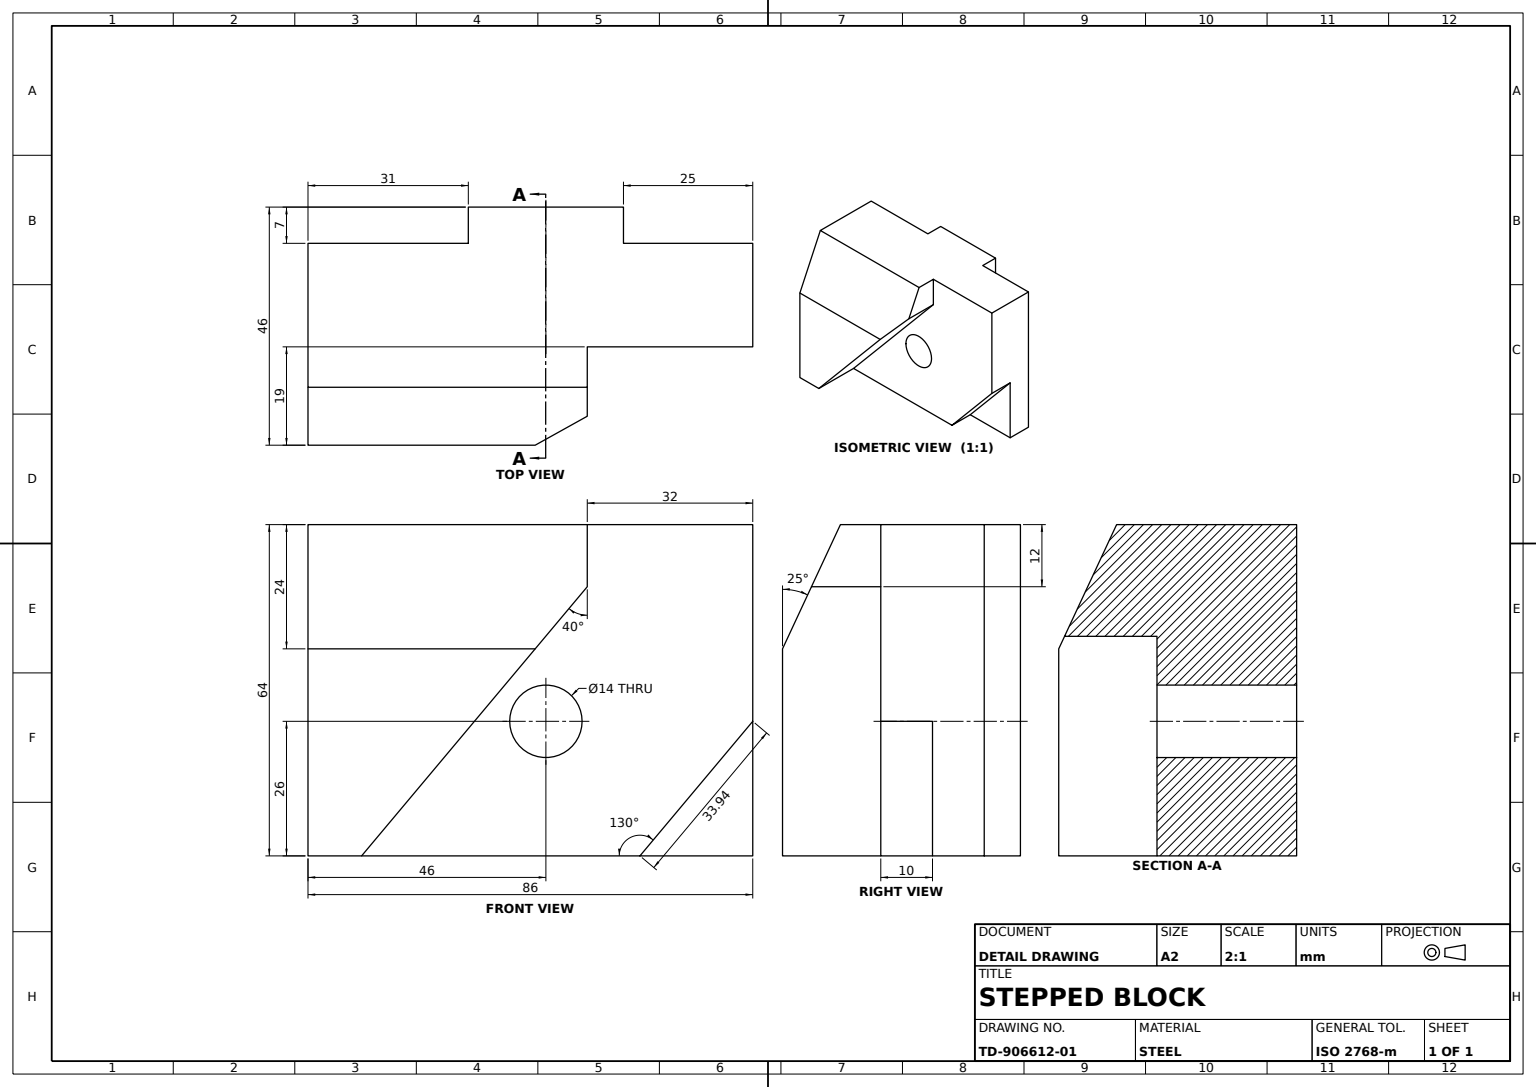
SolidWorks part; units mm, degrees
material "Plain Carbon Steel"
ref_plane "Front Plane" through (0, 0, 0) normal (0, 0, 1) x (1, 0, 0)
ref_plane "Top Plane" through (0, 0, 0) normal (0, 1, 0) x (1, 0, 0)
ref_plane "Right Plane" through (0, 0, 0) normal (1, 0, 0) x (0, 0, -1)
sketch "Base Plate Sketch" plane through (0, 0, 0) normal (0, 0, 1) x (1, 0, 0)
  line L0 (0, 0) -> (0, 64)
  line L1 (0, 64) -> (86, 64)
  line L2 (86, 64) -> (86, 0)
  line L3 (86, 0) -> (0, 0)
  dimension "D1" = 64
  dimension "D2" = 86
  dimension "D3" = 64
extrude "Base Plate 86x64x10" add sketch "Base Plate Sketch" along normal blind 10
sketch "Upper Layer Sketch" plane through (0, 0, 10) normal (0, 0, 1) x (1, 0, 0)
  line L0 (0, 64) -> (0, 0)
  line L1 (0, 0) -> (86, 0)
  line L2 (86, 0) -> (86, 64)
  line L3 (86, 64) -> (0, 64)
extrude "Upper Layer Boss 10" add sketch "Upper Layer Sketch" along normal blind 10
sketch "Angled Step Sketch" plane through (0, 0, 20) normal (0, 0, 1) x (1, 0, 0)
  line L0 (86, 64) -> (54, 64)
  line L1 (86, 64) -> (0, 64) construction
  line L2 (54, 64) -> (54, 52)
  line L3 (0, 64) -> (0, 0)
  line L4 (54, 52) -> (10.3668, 0)
  line L5 (0, 0) -> (10.3668, 0)
  line L6 (0, 0) -> (86, 0) construction
  line L7 (0, 64) -> (54, 64)
  line M3 (86, 64) -> (0, 64)
  line M4 (0, 64) -> (0, 0)
  line M5 (0, 0) -> (86, 0)
  dimension "D1" = 32
  dimension "D2" = 12
  dimension "D3" = 40
extrude "Angled Step Boss 19" add sketch "Angled Step Sketch" along normal blind 19 contours L4 L2 M3 M4 M5
sketch "Angled Cut Sketch" plane through (0, 0, 0) normal (-1, 0, 0) x (0, 0, 1)
  line L0 (39, 64) -> (39, 40)
  line L1 (39, 64) -> (39, 0) construction
  line L2 (39, 40) -> (27.8086, 64)
  line L3 (39, 64) -> (27.8086, 64)
  dimension "D1" = 24
  dimension "D2" = 25
  dimension "D3" = 11.1914
extrude "Angled Cut 25deg" cut sketch "Angled Cut Sketch" against normal blind 65
sketch "Through Hole Sketch" plane through (0, 0, 20) normal (0, 0, 1) x (1, 0, 0)
  line L0 (10.3668, 0) -> (86, 0) construction
  line L1 (0, 40) -> (0, 0) construction
  circle A0 centre (46, 26) radius 7
  dimension "D1" = 14
  dimension "D2" = 26
  dimension "D3" = 46
extrude "Through Hole Ø14" cut sketch "Through Hole Sketch" against normal blind 65
sketch "Triangular Notch Sketch" plane through (0, 0, 20) normal (0, 0, 1) x (1, 0, 0)
  line L0 (86, 0) -> (86, 26)
  line L1 (86, 0) -> (86, 64) construction
  line L4 (86, 26) -> (64.1834, 0)
  line L5 (86, 0) -> (64.1834, 0)
  dimension "D1" = 26
  dimension "D2" = 130
  dimension "D3" = 33.9406
extrude "Triangular Notch Cut" cut sketch "Triangular Notch Sketch" against normal blind 10
sketch "Side Boss Sketch" plane through (0, 0, 0) normal (0, -1, 0) x (1, 0, 0)
  line L0 (31, 0) -> (61, 0)
  line L1 (0, 0) -> (86, 0) construction
  line L2 (61, 0) -> (61, -7)
  line L4 (31, 0) -> (31, -7)
  line L5 (31, -7) -> (61, -7)
  line L6 (86, 10) -> (86, 0) construction
  dimension "D1" = 25
  dimension "D2" = 7
  dimension "D3" = 31
  dimension "D4" = 7
extrude "Side Boss 64" add sketch "Side Boss Sketch" against normal blind 64
sketch "Side Boss Hole Sketch" plane through (0, 0, 0) normal (0, 0, 1) x (1, 0, 0)
  circle A0 centre (46, 26) radius 7
  dimension "D1" = 14
extrude "Side Boss Hole Ø14" cut sketch "Side Boss Hole Sketch" against normal blind 64
